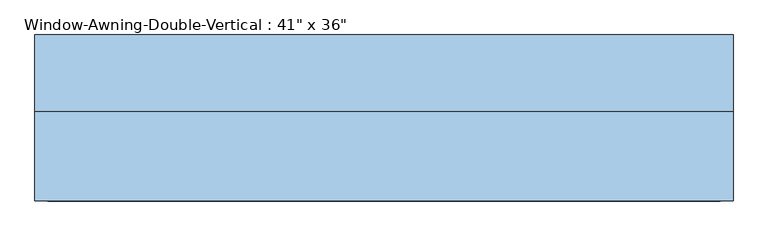
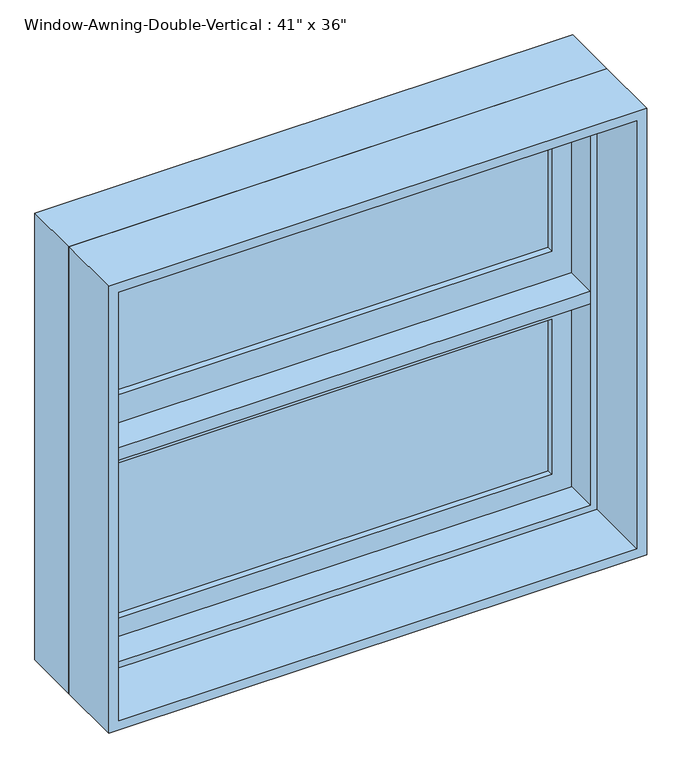
"""IFC4 building model written with IfcOpenShell, lengths in millimetres: window geometry."""

from ifc_helpers import new_model, si_unit, frame, origin, place, context, project, spatial, polyline, outline, extrude, faceted_brep, source, transform, mapped, element, save


def window_fa0038f5(model_context):
    return source(origin(), model_context, "Body", "SolidModel", [
        extrude(outline(polyline([(1828.8, -520.7), (914.4, -520.7), (914.4, 520.7), (1828.8, 520.7), (1828.8, -520.7)]), holes=[polyline([(1809.75, -501.65), (1809.75, 501.65), (933.45, 501.65), (933.45, -501.65), (1809.75, -501.65)])]), frame((0.0, -114.3, 0.0), z_axis=(0.0, 1.0, 0.0), x_axis=(0.0, 0.0, 1.0)), (0.0, 0.0, 1.0), 133.35),
        faceted_brep([(-520.7, 19.05, 1828.8), (-520.7, 133.35, 1828.8), (-520.7, 133.35, 914.4), (-520.7, 19.05, 914.4), (-508.0, 133.35, 1816.1), (-508.0, 82.55, 1816.1), (-508.0, 82.55, 927.1), (-508.0, 133.35, 927.1), (-488.95, 82.55, 1797.05), (-488.95, 19.05, 1797.05), (-488.95, 19.05, 946.15), (-488.95, 82.55, 946.15), (520.7, 133.35, 914.4), (520.7, 19.05, 914.4), (508.0, 82.55, 927.1), (508.0, 133.35, 927.1), (488.95, 19.05, 946.15), (488.95, 82.55, 946.15), (520.7, 133.35, 1828.8), (520.7, 19.05, 1828.8), (508.0, 82.55, 1816.1), (508.0, 133.35, 1816.1), (488.95, 19.05, 1797.05), (488.95, 82.55, 1797.05)], [[[0, 1, 2, 3]], [[4, 5, 6, 7]], [[8, 9, 10, 11]], [[3, 2, 12, 13]], [[7, 6, 14, 15]], [[11, 10, 16, 17]], [[13, 12, 18, 19]], [[15, 14, 20, 21]], [[17, 16, 22, 23]], [[3, 13, 19, 0], [9, 22, 16, 10]], [[19, 18, 1, 0]], [[1, 18, 12, 2], [7, 15, 21, 4]], [[21, 20, 5, 4]], [[5, 20, 14, 6], [11, 17, 23, 8]], [[23, 22, 9, 8]]]),
        extrude(outline(polyline([(1384.3, -508.0), (1384.3, 508.0), (1816.1, 508.0), (1816.1, -508.0), (1384.3, -508.0)]), holes=[polyline([(1758.95, -450.85), (1758.95, 450.85), (1441.45, 450.85), (1441.45, -450.85), (1758.95, -450.85)])]), frame((0.0, 82.55, 0.0), z_axis=(0.0, 1.0, 0.0), x_axis=(0.0, 0.0, 1.0)), (0.0, 0.0, 1.0), 44.45),
        extrude(outline(polyline([(450.85, 114.3), (450.85, 107.95), (-450.85, 107.95), (-450.85, 114.3), (450.85, 114.3)])), frame((0.0, 0.0, 1441.45), z_axis=(0.0, 0.0, 1.0), x_axis=(1.0, 0.0, 0.0)), (0.0, 0.0, 1.0), 317.5),
        extrude(outline(polyline([(450.85, 101.6), (450.85, 95.25), (-450.85, 95.25), (-450.85, 101.6), (450.85, 101.6)])), frame((0.0, 0.0, 1441.45), z_axis=(0.0, 0.0, 1.0), x_axis=(1.0, 0.0, 0.0)), (0.0, 0.0, 1.0), 317.5),
        extrude(outline(polyline([(450.85, 114.3), (450.85, 107.95), (-450.85, 107.95), (-450.85, 114.3), (450.85, 114.3)])), frame((0.0, 0.0, 984.25), z_axis=(0.0, 0.0, 1.0), x_axis=(1.0, 0.0, 0.0)), (0.0, 0.0, 1.0), 317.5),
        extrude(outline(polyline([(450.85, 101.6), (450.85, 95.25), (-450.85, 95.25), (-450.85, 101.6), (450.85, 101.6)])), frame((0.0, 0.0, 984.25), z_axis=(0.0, 0.0, 1.0), x_axis=(1.0, 0.0, 0.0)), (0.0, 0.0, 1.0), 317.5),
        extrude(outline(polyline([(-508.0, 82.55), (-508.0, 133.35), (508.0, 133.35), (508.0, 82.55), (488.95, 82.55), (488.95, 19.05), (-488.95, 19.05), (-488.95, 82.55), (-508.0, 82.55)])), frame((0.0, 0.0, 1358.9), z_axis=(0.0, 0.0, 1.0), x_axis=(1.0, 0.0, 0.0)), (0.0, 0.0, 1.0), 25.4),
        extrude(outline(polyline([(927.1, 508.0), (1358.9, 508.0), (1358.9, -508.0), (927.1, -508.0), (927.1, 508.0)]), holes=[polyline([(984.25, -450.85), (1301.75, -450.85), (1301.75, 450.85), (984.25, 450.85), (984.25, -450.85)])]), frame((0.0, 82.55, 0.0), z_axis=(0.0, 1.0, 0.0), x_axis=(0.0, 0.0, 1.0)), (0.0, 0.0, 1.0), 44.45),
    ])


if __name__ == "__main__":
    model = new_model("IFC4")
    model_context = context("Model", 3, world=origin())
    ifc_project = project(units=[si_unit("LENGTHUNIT", "METRE", prefix="MILLI")], contexts=[model_context])
    site = spatial("IfcSite", under=ifc_project)
    building = spatial("IfcBuilding", under=site)
    placement = place(None, origin())
    window_shape = window_fa0038f5(model_context)
    element("IfcWindow", 1, ObjectType="Window-Awning-Double-Vertical : 41\" x 36\"", at=placement, inside=building, context=model_context, shape_type="MappedRepresentation", body=[
        mapped(window_shape, transform((0.0, 0.0, 0.0), x_axis=(1.0, 0.0, 0.0), y_axis=(0.0, 1.0, 0.0), z_axis=(0.0, 0.0, 1.0))),
    ])
    save(model, "model.ifc")

# Revit data of these elements
# Type "Window-Awning-Double-Vertical : 41\" x 36\""
#   Type Mark = "21"
#   Fire Rating = "0.5h"
#   Assembly Code = "B2020100"
#   Analytic Construction = "Double glazing - domestic"
#   Window Inset [instance default] = 0' - 0"
#   Wall Thickness [instance default] = 0' - 6"
#   Visual Light Transmittance = 0.81
#   Top Sash Height Ratio = 0.5
#   Top Sash Height = 1' - 6"
#   Thermal Resistance (R) = 1.8146 (h·ft²·°F)/BTU
#   Solar Heat Gain Coefficient = 0.76
#   Rough Width = 3' - 5 1/2"
#   Rough Height = 3' - 0 1/2"
#   Interior Wall Closure [instance default] = 0' - 2 1/4"
#   Height = 3' - 0"
#   Heat Transfer Coefficient (U) = 0.5511 BTU/(h·ft²·°F)
#   Frame Extension [instance default] = 0' - 0 1/4"
#   Exterior Wall Closure [instance default] = 0' - 1 1/4"
#   Extension Jamb [instance default] = 0' - 2 1/4"
#   Default Sill Height = 3' - 0"
#   Width = 3' - 5"
#   Top Muntin Visibility = yes
#   Interior Trim Visibility [instance default] = yes
#   Exterior Trim Visibility [instance default] = yes
#   Extension Jamb Visibility [instance default] = yes
#   Bottom Muntin Visibility = yes
#   Muntin Pattern = Muntin Pattern_2x2 : Muntin Pattern_2x2
#   Interior Trim Material = Wood - Stained
#   Interior Trim = Trim-Window-Interior-Flat : Picture Frame
#   Interior Frame Material = Wood - Stained
#   Glass Panel Material = Glass
#   Exterior Trim Material = Clad - White
#   Exterior Trim = Trim-Window-Exterior-Flat : with Sill
#   Exterior Frame Material = Clad - White
#   Wall Closure = (empty or 0)
# Element 1 (IfcWindow, "Window-Awning-Double-Vertical : 41\" x 36\"")
#   Wall Thickness = 0' - 9"
#   Extension Jamb = 0' - 5 1/4"
#   Materials on its faces: "Wood - Stained", "Glass", "Clad - White"
# Materials
#   "Wood - Stained": class "Wood", colour RGB 224 178 126, transparency 0, Cost = 0
#   "Glass": class "Glass", colour RGB 0 128 192, transparency 0.75, Description = "Soda Lime Glass", Cost = 0
#   "Clad - White": class "Wood", colour RGB 242 242 238, transparency 0, Cost = 0
